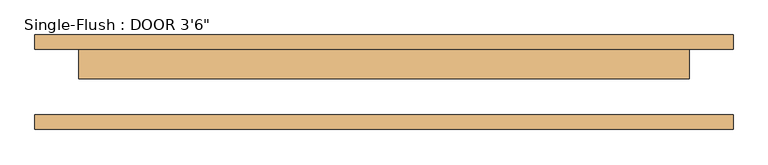
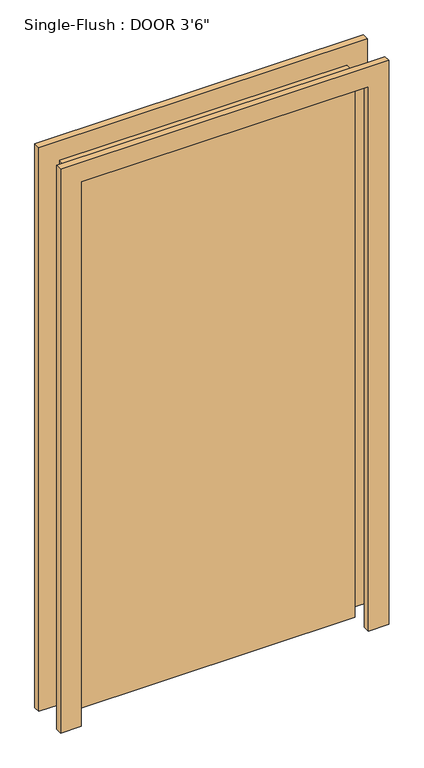
"""IFC4 building model written with IfcOpenShell, lengths in millimetres: door geometry."""

from ifc_helpers import new_model, si_unit, frame, origin, origin_with_axes, place, context, project, spatial, polyline, outline, extrude, source, transform, mapped, element, save


def door_4c162e62(model_context):
    return source(origin(), model_context, "Body", "SweptSolid", [
        extrude(outline(polyline([(2209.8, -609.6), (0.0, -609.6), (0.0, -533.4), (2133.6, -533.4), (2133.6, 533.4), (0.0, 533.4), (0.0, 609.6), (2209.8, 609.6), (2209.8, -609.6)])), frame((0.0, 57.15, 0.0), z_axis=(0.0, 1.0, 0.0), x_axis=(0.0, 0.0, 1.0)), (0.0, 0.0, 1.0), 25.4),
        extrude(outline(polyline([(2209.8, 609.6), (2209.8, -609.6), (0.0, -609.6), (0.0, -533.4), (2133.6, -533.4), (2133.6, 533.4), (0.0, 533.4), (0.0, 609.6), (2209.8, 609.6)])), frame((0.0, -82.55, 0.0), z_axis=(0.0, 1.0, 0.0), x_axis=(0.0, 0.0, 1.0)), (0.0, 0.0, 1.0), 25.4),
        extrude(outline(polyline([(533.4, 6.35), (-533.4, 6.35), (-533.4, 57.15), (533.4, 57.15), (533.4, 6.35)])), origin_with_axes(), (0.0, 0.0, 1.0), 2133.6),
    ])


if __name__ == "__main__":
    model = new_model("IFC4")
    model_context = context("Model", 3, world=origin())
    ifc_project = project(units=[si_unit("LENGTHUNIT", "METRE", prefix="MILLI")], contexts=[model_context])
    site = spatial("IfcSite", under=ifc_project)
    building = spatial("IfcBuilding", under=site)
    placement = place(None, origin())
    door_shape = door_4c162e62(model_context)
    element("IfcDoor", 1, ObjectType="Single-Flush : DOOR 3'6\"", at=placement, inside=building, context=model_context, shape_type="MappedRepresentation", body=[
        mapped(door_shape, transform((0.0, 0.0, 0.0), x_axis=(1.0, 0.0, 0.0), y_axis=(0.0, 1.0, 0.0), z_axis=(0.0, 0.0, 1.0))),
    ])
    save(model, "model.ifc")

# Revit data of these elements
# Type "Single-Flush : DOOR 3'6\""
#   Type Mark = "9"
#   Construction Type Id = "MDOOR"
#   Assembly Code = "C1020"
#   Analytic Construction = "Metal"
#   Thickness = 0' - 2"
#   Heat Transfer Coefficient (U) = 0.651978 BTU/(h·ft²·°F)
#   Height = 7' - 0"
#   Trim Projection Ext = 0' - 1"
#   Trim Projection Int = 0' - 1"
#   Trim Width = 0' - 3"
#   Width = 3' - 6"
#   Define Thermal Properties by = 1
#   Door Material = Door - Panel
#   Frame Material = Door - Frame
#   Visual Light Transmittance = 0
#   Solar Heat Gain Coefficient = 0
#   Function = (empty or 0)
#   Wall Closure = (empty or 0)
# Element 1 (IfcDoor, "Single-Flush : DOOR 3'6\"")
#   Materials on its faces: "Door - Frame", "Door - Panel"
# Materials
#   "Door - Panel": class "Wood", colour RGB 210 159 95, transparency 0, Cost = 0
#   "Door - Frame": colour RGB 118 70 51, transparency 0, Cost = 0
